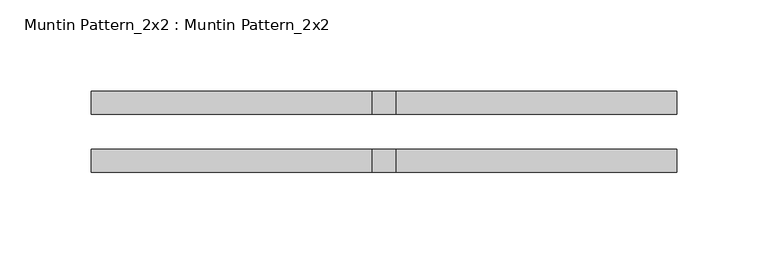
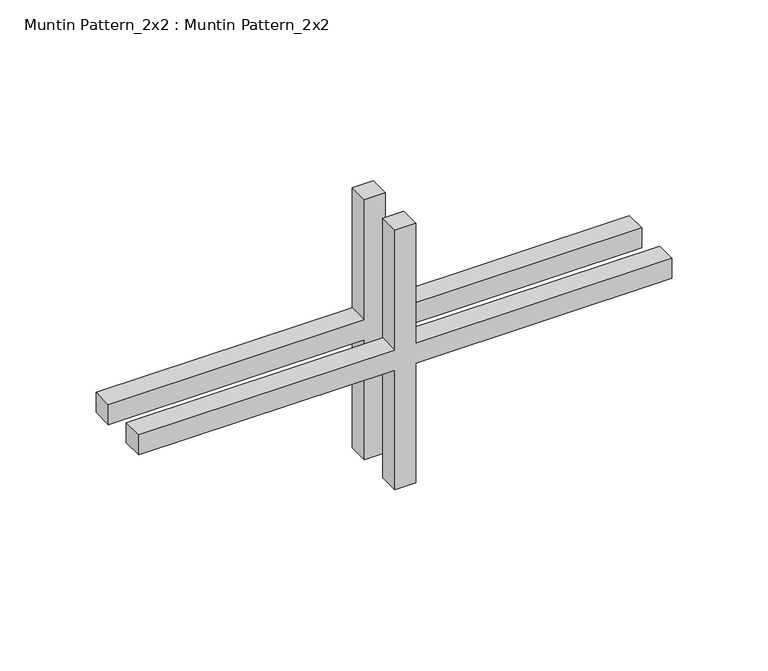
"""IFC4 building model written with IfcOpenShell, lengths in millimetres: proxy geometry, Muntin Pattern_2x2 : Muntin Pattern_2x2."""

from ifc_helpers import new_model, si_unit, frame, origin, place, context, project, spatial, polyline, outline, extrude, source, transform, mapped, element, save


def muntin_pattern_2x2_muntin_pattern_2x2_1c5971db(model_context):
    return source(origin(), model_context, "Body", "SweptSolid", [
        extrude(outline(polyline([(88.9, -6.35), (88.9, -160.3375), (76.2, -160.3375), (76.2, -6.35), (0.0, -6.35), (0.0, 6.35), (76.2, 6.35), (76.2, 160.3375), (88.9, 160.3375), (88.9, 6.35), (165.1, 6.35), (165.1, -6.35), (88.9, -6.35)])), frame((0.0, 9.525, 0.0), z_axis=(0.0, 1.0, 0.0), x_axis=(0.0, 0.0, 1.0)), (0.0, 0.0, 1.0), 12.7),
        extrude(outline(polyline([(88.9, -6.35), (88.9, -160.3375), (76.2, -160.3375), (76.2, -6.35), (0.0, -6.35), (0.0, 6.35), (76.2, 6.35), (76.2, 160.3375), (88.9, 160.3375), (88.9, 6.35), (165.1, 6.35), (165.1, -6.35), (88.9, -6.35)])), frame((0.0, -22.225, 0.0), z_axis=(0.0, 1.0, 0.0), x_axis=(0.0, 0.0, 1.0)), (0.0, 0.0, 1.0), 12.7),
    ])


if __name__ == "__main__":
    model = new_model("IFC4")
    model_context = context("Model", 3, world=origin())
    ifc_project = project(units=[si_unit("LENGTHUNIT", "METRE", prefix="MILLI")], contexts=[model_context])
    site = spatial("IfcSite", under=ifc_project)
    building = spatial("IfcBuilding", under=site)
    placement = place(None, origin())
    muntin_pattern_2x2_muntin_pattern_2x2_shape = muntin_pattern_2x2_muntin_pattern_2x2_1c5971db(model_context)
    element("IfcBuildingElementProxy", 1, Name="Muntin Pattern_2x2 : Muntin Pattern_2x2", ObjectType="Muntin Pattern_2x2 : Muntin Pattern_2x2", at=placement, inside=building, context=model_context, shape_type="MappedRepresentation", body=[
        mapped(muntin_pattern_2x2_muntin_pattern_2x2_shape, transform((0.0, 0.0, 0.0), x_axis=(1.0, 0.0, 0.0), y_axis=(0.0, 1.0, 0.0), z_axis=(0.0, 0.0, 1.0))),
    ])
    save(model, "model.ifc")

# Revit data of these elements
# Type "Muntin Pattern_2x2 : Muntin Pattern_2x2"
#   Width [instance default] = 4' - 0"
#   Thickness = 0' - 0 1/2"
#   Height [instance default] = 4' - 0"
#   Distance = 0' - 0 3/4"
#   Interior Material [instance default] = none
#   Exterior Material [instance default] = none
#   Default Elevation = 0
# Element 1 (IfcBuildingElementProxy, "Muntin Pattern_2x2 : Muntin Pattern_2x2")
#   Width = 1' - 0 5/8"
#   Height = 0' - 6 1/2"
#   Interior Material = Wood - Stained
#   Exterior Material = Clad - White
#   Materials on its faces: "Clad - White", "Wood - Stained"
# Materials
#   "Clad - White": class "Wood", colour RGB 242 242 238, transparency 0, Cost = 0
#   "Wood - Stained": class "Wood", colour RGB 224 178 126, transparency 0, Cost = 0
